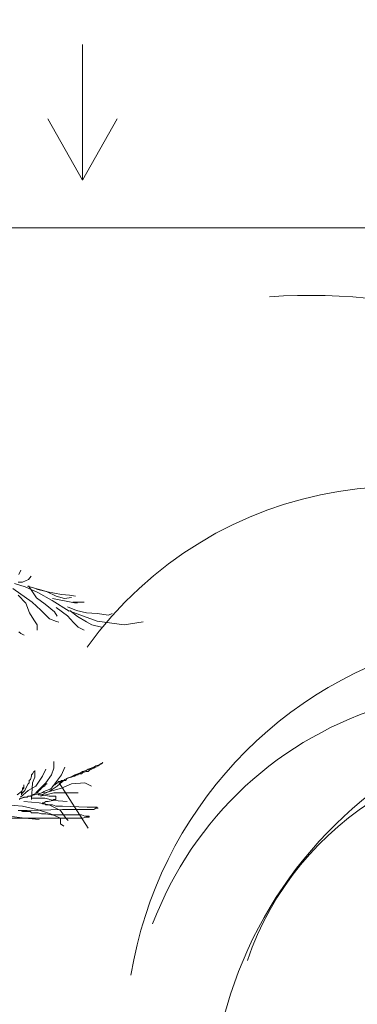
# Model space of a CAD drawing. Units: millimetres. Extents: x 595116 to 630915, y 909473 to 920225.
# Tile 28 of 134: x 629613 to 629622, y 919165 to 919190. Entities that reach past the tile are written whole.
import ezdxf

# ---------------------------------------------------------------- set-up
doc = ezdxf.new("R2010")
doc.units = ezdxf.units.MM
doc.layers.add('Dimension', color=3, linetype='Continuous', lineweight=18)
doc.layers.add('L-PLNT', color=85, linetype='Continuous', lineweight=13)
doc.styles.get("Standard").update_dxf_attribs({"font": 'arial.ttf'})
doc.dimstyles.new('ISO-25', dxfattribs={"dimtxt": 9, "dimasz": 6, "dimexe": 1.25, "dimexo": 0.625, "dimtad": 1, "dimlunit": 4, "dimtxsty": 'Standard', "dimcen": 2.5, "dimadec": 0, "dimazin": 0, "dimtfac": 1, "dimtmove": 0, "dimatfit": 3, "dimfxl": 1, "dimarcsym": 0})

# ---------------------------------------------------------------- blocks, each defined once
blk = doc.blocks.new('tree')
for centre, radius, start, end in [((629594.259, 919292.132), 6.965, 7.4001, 94.0059), ((629595.377, 919292.044), 4.722, 54.2484, 144.2167), ((629597.025, 919289.989), 5.01, 36.0581, 170.6542), ((629596.464, 919289.874), 4.4, 52.9074, 159.3471), ((629598.153, 919288.998), 5.103, 105.3576, 208.8973), ((629597.068, 919289.758), 3.768, 80.4816, 161.0664)]:
    blk.add_arc(centre, radius, start, end)
blk = doc.blocks.new('A$C4FB75ABC')
for p, q in [((4.5963, 3.4774), (4.6082, 3.5072)), ((4.6201, 3.4238), (4.6619, 3.4416)), ((4.6619, 3.4416), (4.6798, 3.4655)), ((4.5545, 3.382), (4.6858, 3.2866)), ((4.5657, 3.4153), (4.6395, 3.3917)), ((4.5903, 3.4238), (4.6201, 3.4238)), ((4.6395, 3.3917), (4.7247, 3.3534)), ((4.6551, 3.396), (4.7847, 3.3597)), ((4.6619, 3.3999), (4.7156, 3.3164)), ((4.7156, 3.3761), (4.7931, 3.3582)), ((4.5903, 3.3343), (4.644, 3.2807)), ((4.7156, 3.3164), (4.7752, 3.2747)), ((4.7247, 3.3534), (4.8242, 3.2989)), ((4.7847, 3.3597), (4.8521, 3.3286)), ((4.7931, 3.3582), (4.8886, 3.3403)), ((4.8262, 3.3131), (4.9765, 3.282)), ((4.8521, 3.3286), (4.9091, 3.3131)), ((4.8886, 3.3403), (4.9422, 3.3343)), ((4.9091, 3.3131), (4.9558, 3.3183)), ((4.9422, 3.3343), (4.984, 3.3284)), ((4.644, 3.2807), (4.6679, 3.2151)), ((4.6858, 3.2866), (4.7454, 3.233)), ((4.7752, 3.2747), (4.8408, 3.2211)), ((4.8242, 3.2989), (4.9411, 3.2265)), ((4.8521, 3.2509), (4.9299, 3.1939)), ((4.9299, 3.2561), (4.9921, 3.2302)), ((4.9661, 3.2866), (5.0079, 3.2866)), ((4.9765, 3.282), (4.9973, 3.282)), ((5.0079, 3.2866), (5.0437, 3.2866)), ((4.6679, 3.2151), (4.6977, 3.1674)), ((4.7454, 3.233), (4.8051, 3.1734)), ((4.8051, 3.1734), (4.8528, 3.1555)), ((4.8408, 3.2211), (4.8587, 3.1912)), ((4.9299, 3.1939), (4.9713, 3.1472)), ((4.9454, 3.2302), (4.9973, 3.1887)), ((4.9454, 3.225), (5.1321, 3.1576)), ((4.9921, 3.2302), (5.0595, 3.2146)), ((4.9973, 3.1887), (5.0595, 3.1524)), ((5.0595, 3.2146), (5.1321, 3.2094)), ((5.1321, 3.2094), (5.2099, 3.1991)), ((5.2099, 3.1991), (5.2358, 3.2094)), ((4.6977, 3.1674), (4.7215, 3.1316)), ((4.7215, 3.1316), (4.7215, 3.0959)), ((4.8528, 3.1555), (4.8707, 3.1495)), ((4.9713, 3.1472), (5.0025, 3.1162)), ((5.0025, 3.1162), (5.0439, 3.0954)), ((5.0595, 3.1524), (5.0958, 3.1317)), ((5.0958, 3.1317), (5.1632, 3.1162)), ((5.1321, 3.1576), (5.3187, 3.1317)), ((5.3187, 3.1317), (5.4484, 3.1524)), ((4.5963, 3.0839), (4.6082, 3.072)), ((4.6082, 3.072), (4.6321, 3.0601)), ((4.835, 2.1495), (4.835, 2.1952)), ((5.1248, 2.1648), (5.1095, 2.1571)), ((5.1477, 2.1724), (5.1248, 2.1648)), ((5.1248, 2.1571), (5.1401, 2.1648)), ((5.1401, 2.1648), (5.1477, 2.1724)), ((5.1477, 2.1724), (5.1629, 2.18)), ((5.1553, 2.18), (5.1477, 2.1724)), ((5.1706, 2.1876), (5.1553, 2.18)), ((5.1629, 2.18), (5.1706, 2.1876)), ((4.6749, 2.0733), (4.6825, 2.0961)), ((4.6825, 2.1038), (4.6901, 2.1114)), ((4.6825, 2.0961), (4.6825, 2.1038)), ((4.6901, 2.1114), (4.6977, 2.1266)), ((4.6977, 2.1266), (4.7054, 2.1266)), ((4.7054, 2.1266), (4.7054, 2.1343)), ((4.7054, 2.1343), (4.7054, 2.0885)), ((4.713, 2.0275), (4.7587, 2.0961)), ((4.7587, 2.0961), (4.7816, 2.1419)), ((4.7816, 2.0504), (4.8198, 2.1038)), ((4.8121, 2.0047), (4.8884, 2.1038)), ((4.8198, 2.1038), (4.835, 2.1495)), ((4.8884, 2.1038), (4.9113, 2.1571)), ((4.9113, 2.0733), (5.079, 2.1419)), ((4.9799, 2.1038), (4.9494, 2.0885)), ((4.957, 2.0885), (4.9723, 2.0961)), ((4.9723, 2.0961), (4.9799, 2.0961)), ((5.018, 2.119), (4.9799, 2.1038)), ((4.9799, 2.0961), (4.9952, 2.1038)), ((4.9952, 2.1038), (5.0028, 2.1038)), ((5.0028, 2.1038), (5.0028, 2.1114)), ((5.0028, 2.1114), (5.0257, 2.1114)), ((5.0333, 2.1266), (5.018, 2.119)), ((5.0257, 2.1114), (5.0333, 2.119)), ((5.0562, 2.1343), (5.0333, 2.1266)), ((5.0333, 2.119), (5.0562, 2.1266)), ((5.0714, 2.1419), (5.0562, 2.1343)), ((5.0562, 2.1266), (5.0714, 2.1266)), ((5.1095, 2.1571), (5.0714, 2.1419)), ((5.0714, 2.1266), (5.079, 2.1343)), ((5.079, 2.1343), (5.0867, 2.1419)), ((5.0867, 2.1419), (5.0943, 2.1419)), ((5.0943, 2.1419), (5.1019, 2.1495)), ((5.1019, 2.1495), (5.1095, 2.1495)), ((5.1095, 2.1495), (5.1172, 2.1571)), ((5.1172, 2.1571), (5.1248, 2.1571)), ((4.6291, 2.0199), (4.6291, 2.0352)), ((4.6291, 2.0352), (4.6291, 2.0123)), ((4.6444, 2.0123), (4.6596, 2.0428)), ((4.6596, 2.0428), (4.6672, 2.0504)), ((4.6596, 1.9971), (4.713, 2.0275)), ((4.6672, 2.0657), (4.6749, 2.0733)), ((4.6672, 2.0504), (4.6672, 2.0657)), ((4.6901, 2.0504), (4.6825, 1.9361)), ((4.6977, 2.0733), (4.6901, 2.0504)), ((4.7054, 2.0885), (4.6977, 2.0733)), ((4.713, 1.9818), (4.7816, 2.0504)), ((4.7664, 2.0275), (4.7511, 2.0123)), ((4.774, 2.0275), (4.7664, 2.0275)), ((4.7816, 2.0352), (4.774, 2.0352)), ((4.774, 2.0352), (4.774, 2.0275)), ((4.7892, 2.0428), (4.7816, 2.0428)), ((4.7816, 2.0428), (4.7816, 2.0352)), ((4.8045, 1.9894), (4.8579, 2.0275)), ((4.8198, 2.0123), (4.8274, 2.0275)), ((4.8274, 2.0275), (4.8426, 2.0352)), ((4.8426, 2.0352), (4.8579, 2.0504)), ((4.8579, 2.0275), (4.9113, 2.0733)), ((4.8579, 2.0504), (4.8655, 2.0504)), ((4.8655, 2.0504), (4.8655, 2.058)), ((4.8655, 2.058), (4.8808, 2.058)), ((4.8808, 2.0504), (4.8731, 2.0504)), ((4.8731, 2.0504), (5.0714, 1.7379)), ((4.8808, 2.058), (4.8884, 2.0657)), ((4.896, 2.058), (4.8808, 2.058)), ((4.8808, 2.058), (4.8808, 2.0504)), ((4.8884, 2.0657), (4.9036, 2.0657)), ((4.8884, 2.0123), (4.957, 2.0428)), ((4.9036, 2.0657), (4.896, 2.058)), ((4.9036, 2.0657), (4.9113, 2.0733)), ((4.9189, 2.0657), (4.9036, 2.0657)), ((4.9113, 2.0733), (4.9265, 2.0809)), ((4.9265, 2.0809), (4.9189, 2.0657)), ((4.9265, 2.0809), (4.957, 2.0885)), ((4.9494, 2.0885), (4.9265, 2.0809)), ((4.957, 2.0428), (5.0485, 2.0504)), ((5.0485, 2.0504), (5.0943, 2.0275)), ((4.5833, 1.9666), (4.6138, 1.9894)), ((4.7725, 1.9851), (4.5975, 1.9398)), ((4.6062, 1.9513), (4.6596, 1.9971)), ((4.6138, 1.9894), (4.6215, 2.0047)), ((4.6215, 2.0047), (4.6138, 1.9818)), ((4.6138, 1.9818), (4.6138, 1.9666)), ((4.6138, 1.9742), (4.6215, 1.9818)), ((4.6138, 1.9666), (4.6138, 1.9742)), ((4.6215, 2.0123), (4.6291, 2.0199)), ((4.6215, 2.0047), (4.6215, 2.0123)), ((4.6291, 2.0123), (4.6215, 2.0047)), ((4.6215, 1.9818), (4.6367, 1.9971)), ((4.6367, 1.9971), (4.6444, 2.0123)), ((4.6596, 1.9589), (4.652, 1.9513)), ((4.6825, 1.9589), (4.6596, 1.9589)), ((4.6901, 1.9666), (4.6825, 1.9589)), ((4.7054, 1.9742), (4.6901, 1.9666)), ((4.7206, 1.9818), (4.7054, 1.9742)), ((4.7359, 1.9971), (4.7206, 1.9818)), ((4.7282, 1.9666), (4.7282, 1.9742)), ((4.7282, 1.9742), (4.7359, 1.9742)), ((4.7587, 1.9666), (4.7282, 1.9666)), ((4.7435, 2.0047), (4.7359, 1.9971)), ((4.7359, 1.9742), (4.7511, 1.9818)), ((4.7511, 2.0123), (4.7435, 2.0047)), ((4.7435, 1.9589), (4.835, 1.9818)), ((4.7511, 1.9818), (4.7664, 1.9894)), ((4.7511, 1.9666), (4.8045, 1.9894)), ((4.8045, 1.9589), (4.7587, 1.9666)), ((4.7664, 1.9894), (4.8045, 2.0047)), ((4.774, 1.9818), (4.8884, 2.0123)), ((4.8045, 2.0047), (4.8198, 2.0123)), ((4.8503, 1.9589), (4.8045, 1.9589)), ((4.835, 1.9818), (4.9494, 1.9818)), ((4.8503, 1.9361), (4.8503, 1.9589)), ((4.9494, 1.9818), (5.0028, 1.9818)), ((4.5071, 1.898), (4.6215, 1.8903)), ((4.6138, 1.9437), (4.5986, 1.9361)), ((4.6291, 1.9513), (4.6138, 1.9437)), ((4.6215, 1.8903), (4.7206, 1.8675)), ((4.652, 1.9513), (4.6291, 1.9513)), ((4.6291, 1.9208), (4.7359, 1.9132)), ((4.6825, 1.9437), (4.774, 1.9437)), ((4.7359, 1.9132), (4.8045, 1.898)), ((4.7587, 1.9056), (4.7587, 1.9132)), ((4.7587, 1.9132), (4.7664, 1.9132)), ((4.774, 1.9056), (4.7587, 1.9056)), ((4.7664, 1.9132), (4.7816, 1.9208)), ((4.774, 1.9437), (4.835, 1.9285)), ((4.7816, 1.898), (4.774, 1.9056)), ((4.7816, 1.9208), (4.7969, 1.9208)), ((4.8274, 1.898), (4.7816, 1.898)), ((4.7969, 1.9208), (4.8274, 1.9285)), ((4.8045, 1.898), (4.8808, 1.8599)), ((4.8274, 1.9285), (4.835, 1.9361)), ((4.8503, 1.8903), (4.8274, 1.898)), ((4.835, 1.9361), (4.8503, 1.9361)), ((4.835, 1.9285), (4.9265, 1.9208)), ((4.896, 1.8903), (4.8503, 1.8903)), ((5.0638, 1.8827), (4.896, 1.8903)), ((4.53, 1.8217), (4.6367, 1.8065)), ((4.6062, 1.8599), (4.591, 1.8599)), ((4.591, 1.8599), (4.652, 1.8599)), ((4.6215, 1.8522), (4.6062, 1.8599)), ((4.6749, 1.8522), (4.6215, 1.8522)), ((4.652, 1.8599), (4.896, 1.8675)), ((4.6825, 1.8446), (4.6749, 1.8522)), ((4.7282, 1.8446), (4.6825, 1.8446)), ((4.7206, 1.8675), (4.8121, 1.837)), ((4.7511, 1.837), (4.7282, 1.8446)), ((4.7816, 1.837), (4.7511, 1.837)), ((4.8198, 1.8294), (4.7816, 1.837)), ((4.8121, 1.837), (4.8808, 1.8065)), ((5.0257, 1.8294), (4.8198, 1.8294)), ((4.8808, 1.8599), (4.9189, 1.8065)), ((4.896, 1.8675), (5.1095, 1.8675)), ((5.0485, 1.8217), (5.0257, 1.8294)), ((5.079, 1.8217), (5.0485, 1.8217)), ((5.1324, 1.8827), (5.0638, 1.8827)), ((5.079, 1.8141), (5.079, 1.8217)), ((5.1095, 1.8675), (5.1248, 1.8751)), ((5.1248, 1.8751), (5.1401, 1.8751)), ((5.1324, 1.8751), (5.1324, 1.8827)), ((5.1401, 1.8751), (5.1324, 1.8751)), ((4.1639, 1.8065), (5.0333, 1.8065)), ((4.6367, 1.8065), (4.7359, 1.7989)), ((4.8808, 1.8065), (4.8808, 1.7684)), ((4.8808, 1.7684), (4.9036, 1.7531)), ((4.9189, 1.8065), (4.9341, 1.7913)), ((5.0333, 1.8065), (5.0562, 1.8141)), ((5.0562, 1.8141), (5.079, 1.8141))]:
    blk.add_line(p, q)
blk = doc.blocks.new('LAWN-GRASS-TUFT')
blk.add_line((0.892, 3.485), (0.892, 0))
blk.add_lwpolyline([(0, 1.577), (0.892, 0), (1.785, 1.577)])
blk = doc.blocks.new('*D216')
at = {"layer": 'Defpoints', "color": 0, "transparency": 16777216}
for p in [(629743.541, 919411.928), (629505.041, 919411.828), (629743.541, 918832.378)]:
    blk.add_point(p, dxfattribs=at)
at = {"layer": 'Dimension', "color": 0, "lineweight": -2, "transparency": 16777216}
for p, q in [((629505.041, 919411.203), (629505.041, 918831.128)), ((629743.541, 919411.303), (629743.541, 918831.128)), ((629511.041, 918832.378), (629737.541, 918832.378))]:
    blk.add_line(p, q, dxfattribs=at)
at = {"layer": 'Dimension', "color": 0, "transparency": 16777216}
for points in [[(629511.041, 918833.378), (629511.041, 918831.378), (629505.041, 918832.378)], [(629737.541, 918833.378), (629737.541, 918831.378), (629743.541, 918832.378)]]:
    blk.add_solid(points, dxfattribs=at)
at = {"layer": 'Dimension', "color": 0, "transparency": 16777216, "insert": (629624.291, 918837.656), "char_height": 9, "attachment_point": 5}
blk.add_mtext('19\'-10 1/2"', dxfattribs=at)

msp = doc.modelspace()

# ---------------------------------------------------------------- linework, layer by layer
at = {"layer": 'L-PLNT'}
msp.add_line((629535.274, 919184.917), (629800.951, 919184.917), dxfattribs=at)

# ---------------------------------------------------------------- block references
msp.add_blockref('LAWN-GRASS-TUFT', (629613.938, 919186.14), dxfattribs=at)
for name, p, xscale, yscale, zscale in [('tree', (-697368.484, -1018413.796), 2.107689410566463, 2.107689410566463, 2.107689410566463), ('A$C4FB75ABC', (629595.944, 919162.946), 3.753413438031968, 3.753413438031968, 3.753413438031968)]:
    msp.add_blockref(name, p, dxfattribs=dict(at, xscale=xscale, yscale=yscale, zscale=zscale))

# ---------------------------------------------------------------- dimensions: what is measured, and where the dimension line sits
at = {"layer": 'Dimension'}
dim = msp.add_linear_dim(base=(629743.541, 918832.378), p1=(629505.041, 919411.828), p2=(629743.541, 919411.928), dimstyle='ISO-25', override={"dimdec": 1, "dimlfac": 1, "dimrnd": 0, "dimzin": 1, "dimdsep": 46, "dimlunit": 4, "dimfrac": 2}, dxfattribs=at)
dim.commit()
dim.dimension.update_dxf_attribs({"geometry": '*D216', "text_midpoint": (629624.291, 918837.656)})

doc.saveas('drawing.dxf')
